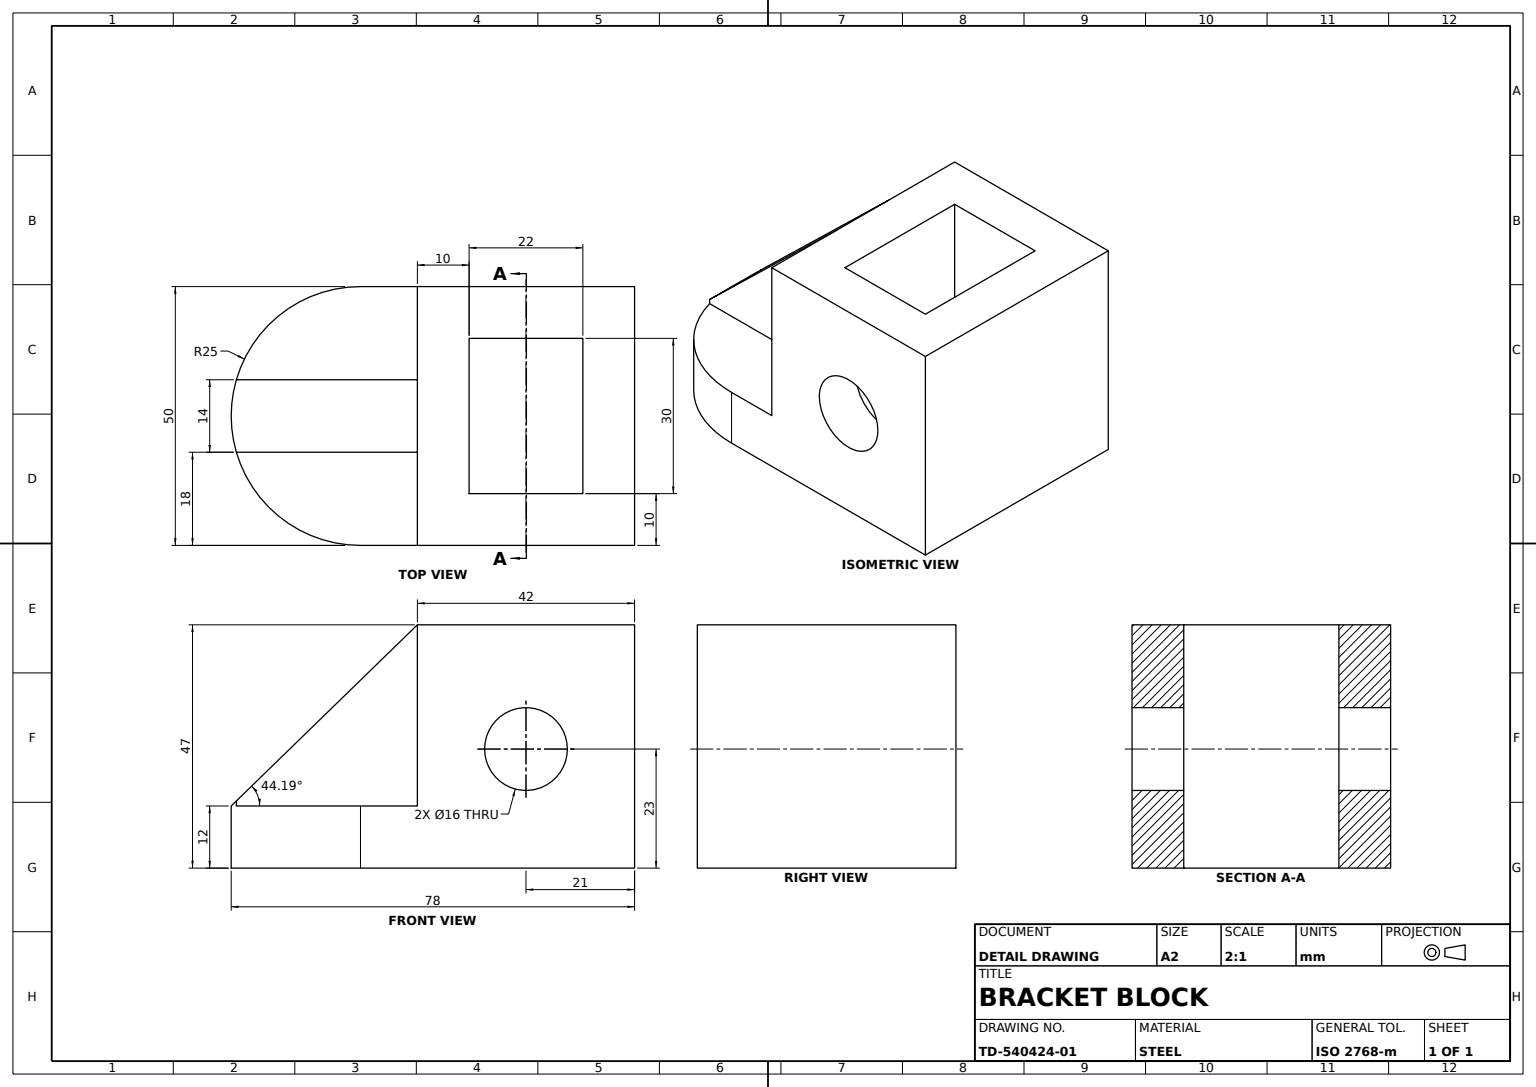
SolidWorks part; units mm, degrees
material "Plain Carbon Steel"
ref_plane "Front Plane" through (0, 0, 0) normal (0, 0, 1) x (1, 0, 0)
ref_plane "Top Plane" through (0, 0, 0) normal (0, 1, 0) x (1, 0, 0)
ref_plane "Right Plane" through (0, 0, 0) normal (1, 0, 0) x (0, 0, -1)
sketch "Base Plate Sketch" plane through (0, 0, 0) normal (1, 0, 0) x (0, 0, -1)
  line L1 (-39, -6) -> (39, -6)
  line L2 (-39, -6) -> (-39, 6)
  line L3 (-39, 6) -> (39, 6)
  line L4 (39, -6) -> (39, 6)
  line L5 (-39, -6) -> (39, 6) construction
  line L6 (-39, 6) -> (39, -6) construction
  point P0 (0, 0)
  dimension "D1" = 78
  dimension "D2" = 12
extrude "Base Plate" add sketch "Base Plate Sketch" against normal blind 50
sketch "Upright Block Sketch" plane through (0, 0, 0) normal (1, 0, 0) x (0, 0, -1)
  line L0 (39, 6) -> (-39, 6) construction
  line L1 (39, 6) -> (-3, 6)
  line L2 (39, 6) -> (39, 41)
  line L3 (39, 41) -> (-3, 41)
  line L4 (-3, 6) -> (-3, 41)
  dimension "D1" = 35
  dimension "D2" = 42
  dimension "D5" = 3
extrude "Upright Block" add sketch "Upright Block Sketch" against normal blind 50
sketch "Block Pocket Sketch" plane through (0, 41, 0) normal (0, 1, 0) x (1, 0, 0)
  line L0 (-25, 39) -> (-25, -3) construction
  line L1 (-50, 39) -> (0, 39) construction
  line L2 (-50, -3) -> (0, -3) construction
  line L3 (-50, 18) -> (0, 18) construction
  line L4 (-50, 39) -> (-50, -3) construction
  line L5 (0, 39) -> (0, -3) construction
  line L7 (-40, 29) -> (-10, 29)
  line L8 (-40, 29) -> (-40, 7)
  line L9 (-40, 7) -> (-10, 7)
  line L10 (-10, 29) -> (-10, 7)
  line L11 (-40, 29) -> (-10, 7) construction
  line L12 (-40, 7) -> (-10, 29) construction
  point P12 (-25, 18)
  dimension "D1" = 30
  dimension "D2" = 22
extrude "Block Pocket 30x22" cut sketch "Block Pocket Sketch" against normal through all
sketch "Side Cut 1 Sketch" plane through (0, 0, 0) normal (1, 0, 0) x (0, 0, -1)
  line L0 (18, 48.1127) -> (18, -15.4182) construction
  line L1 (-16.5231, 17) -> (48.4248, 17) construction
  line L2 (39, -6) -> (39, 41) construction
  line L4 (-39, -6) -> (39, -6) construction
  circle A0 centre (18, 17) radius 8
  dimension "D3" = 16
  dimension "D1" = 21
  dimension "D2" = 23
extrude "Side Cut 1" cut sketch "Side Cut 1 Sketch" against normal blind 10
sketch "Side Cut 2 Sketch" plane through (-50, 0, 0) normal (-1, 0, 0) x (0, 0, 1)
  line L0 (-18, 46.0112) -> (-18, -13.4209) construction
  line L1 (-49.9537, 17) -> (14.6081, 17) construction
  line L2 (-39, -6) -> (-39, 41) construction
  line L3 (39, -6) -> (-39, -6) construction
  circle A0 centre (-18, 17) radius 8
  dimension "D3" = 16
  dimension "D1" = 21
  dimension "D2" = 23
extrude "Side Cut 2" cut sketch "Side Cut 2 Sketch" against normal blind 10
ref_plane "Rib Plane" through (-25, 0, 0) normal (1, 0, 0) x (0, 0, -1)
sketch "Gusset Rib Sketch" plane through (-25, 0, 0) normal (1, 0, 0) x (0, 0, -1)
  line L0 (-39, 6) -> (-3, 41)
rib "Gusset Rib 14mm" sketch "Gusset Rib Sketch" sketch "Gusset Rib Sketch" thickness 14 extrusion direction parallel to sketch draft on no parameters "D1"=14
sketch "Front Profile Cut Sketch" plane through (0, 6, 0) normal (0, 1, 0) x (1, 0, 0)
  line L0 (-57.748, -14) -> (7.748, -14) construction
  line L1 (-18, -39) -> (0, -39) construction
  line L2 (-50, -39) -> (0, -39)
  line L3 (-50, -3) -> (-50, -39) construction
  line L5 (-50, -14) -> (-50, -39)
  line L6 (0, -14) -> (0, -39)
  arc A0 (-50, -14) -> (0, -14) centre (-25, -14) ccw
  line M3 (-18, -3) -> (-18, -39)
  line M4 (-18, -39) -> (0, -39)
  line M5 (0, -39) -> (0, -3)
  dimension "D1" = 25
extrude "Front Profile Cut" cut sketch "Front Profile Cut Sketch" against normal through all contours A0 L5 L2 | A0 M3 M4 M5
sketch "Rib Trim Cut Sketch" plane through (0, -6, 0) normal (0, -1, 0) x (1, 0, 0)
  line L0 (-32, 39) -> (-32, 38)
  line L1 (-32, 39) -> (-25, 39)
  line L5 (-18, 39) -> (-25, 39)
  line L6 (-50, 14) -> (-50, -39)
  line L7 (-50, -39) -> (0, -39)
  line L8 (0, -39) -> (0, 14)
  line L9 (-18, 38) -> (-18, 39)
  line L10 (-18, 39) -> (-25, 39)
  line L11 (-50, 14) -> (-50, -39)
  line L12 (-50, -39) -> (0, -39)
  line L13 (0, -39) -> (0, 14)
  line L14 (-18, 38) -> (-18, 39)
  arc A2 (-25, 39) -> (-50, 14) centre (-25, 14) ccw
  arc A3 (0, 14) -> (-18, 38) centre (-25, 14) ccw
  arc A4 (-25, 39) -> (-32, 38) centre (-25, 14) ccw
  arc A5 (-18, 38) -> (-25, 39) centre (-25, 14) ccw
  arc M13 (-25, 39) -> (-50, 14) centre (-25, 14) ccw
  dimension "D1" = 0
extrude "Rib Trim Cut" cut sketch "Rib Trim Cut Sketch" against normal blind 20 contours L1 L0 M13 | A5 L14 L10
